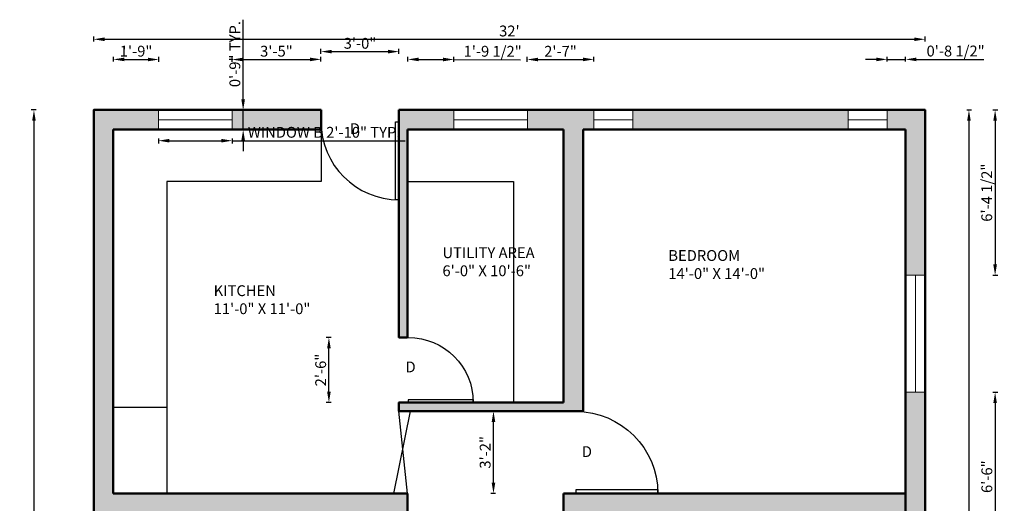
# Model space of a CAD drawing. Units: inches. Extents: x -41 to 449, y -587 to 56.
# Tile 2 of 2: x -32 to 422, y -167 to 56. Entities that reach past the tile are written whole.
import ezdxf

# ---------------------------------------------------------------- set-up
doc = ezdxf.new("R2010")
doc.units = ezdxf.units.IN
for name, color, linetype, lineweight in [('A-ANNO-DIMS', 2, 'Continuous', 18), ('A-ANNO-TEXT', 7, 'Continuous', 18), ('A-AREA-IDEN', 7, 'Continuous', 25), ('A-DOOR', 3, 'Continuous', 25), ('A-FLOR-CASE', 8, 'Continuous', 25), ('A-GLAZ', 4, 'Continuous', 18), ('A-WALL', 7, 'Continuous', 50), ('A-WALL-PATT', 252, 'Continuous', 13)]:
    doc.layers.add(name, color=color, linetype=linetype, lineweight=lineweight)
doc.styles.get("Standard").update_dxf_attribs({"font": 'arial.ttf'})
doc.dimstyles.new('ISO-25', dxfattribs={"dimtxt": 5, "dimasz": 5, "dimexe": 1.25, "dimexo": 0.625, "dimtad": 1, "dimlunit": 3, "dimtxsty": 'Standard', "dimcen": 2.5, "dimadec": 0, "dimazin": 0, "dimtfac": 1, "dimtmove": 0, "dimatfit": 3, "dimfxl": 1, "dimfxlon": 1, "dimarcsym": 0})

# ---------------------------------------------------------------- blocks, each defined once
blk = doc.blocks.new('*U2')
for p, q in [((0, 0), (0, -6)), ((40, 0), (40, -6))]:
    blk.add_line(p, q)
blk.add_lwpolyline([(0, 0), (0, 40), (1.75, 40), (1.75, 0)], close=True)
blk.add_arc((0, 0), 40, 0, 90)
blk = doc.blocks.new('*D3')
at = {"layer": 'A-ANNO-DIMS', "color": 0, "lineweight": -2, "transparency": 16777216}
for p, q in [((1.69, 45.8), (1.69, 48.05)), ((6.69, 46.8), (380.69, 46.8)), ((385.69, 45.8), (385.69, 48.05))]:
    blk.add_line(p, q, dxfattribs=at)
at = {"layer": 'A-ANNO-DIMS', "color": 0, "transparency": 16777216}
for points in [[(6.69, 47.63), (6.69, 45.97), (1.69, 46.8)], [(380.69, 47.63), (380.69, 45.97), (385.69, 46.8)]]:
    blk.add_solid(points, dxfattribs=at)
at = {"layer": 'Defpoints', "color": 0, "transparency": 16777216}
for p in [(385.69, 46.8), (1.69, 14.17), (385.69, 14.17)]:
    blk.add_point(p, dxfattribs=at)
at = {"layer": 'A-ANNO-DIMS', "color": 0, "transparency": 16777216, "insert": (193.69, 49.98), "char_height": 5, "attachment_point": 5}
blk.add_mtext("32'", dxfattribs=at)
blk = doc.blocks.new('*D4')
at = {"layer": 'A-ANNO-DIMS', "color": 0, "lineweight": -2, "transparency": 16777216}
for p, q in [((404.95, 14.17), (407.2, 14.17)), ((405.95, 9.17), (405.95, -524.83)), ((404.95, -529.83), (407.2, -529.83))]:
    blk.add_line(p, q, dxfattribs=at)
at = {"layer": 'A-ANNO-DIMS', "color": 0, "transparency": 16777216}
for points in [[(405.11, 9.17), (406.78, 9.17), (405.95, 14.17)], [(405.11, -524.83), (406.78, -524.83), (405.95, -529.83)]]:
    blk.add_solid(points, dxfattribs=at)
at = {"layer": 'Defpoints', "color": 0, "transparency": 16777216}
for p in [(385.69, 14.17), (385.69, -529.83), (405.95, -529.83)]:
    blk.add_point(p, dxfattribs=at)
at = {"layer": 'A-ANNO-DIMS', "color": 0, "transparency": 16777216, "insert": (402.78, -257.83), "char_height": 5, "attachment_point": 5, "rotation": 90}
blk.add_mtext('45\'-4"', dxfattribs=at)
blk = doc.blocks.new('*D5')
at = {"layer": 'A-ANNO-DIMS', "color": 0, "lineweight": -2, "transparency": 16777216}
for p, q in [((-24.91, 14.17), (-27.16, 14.17)), ((-25.91, 9.17), (-25.91, -454.83)), ((-24.91, -459.83), (-27.16, -459.83))]:
    blk.add_line(p, q, dxfattribs=at)
at = {"layer": 'A-ANNO-DIMS', "color": 0, "transparency": 16777216}
for points in [[(-26.74, 9.17), (-25.07, 9.17), (-25.91, 14.17)], [(-26.74, -454.83), (-25.07, -454.83), (-25.91, -459.83)]]:
    blk.add_solid(points, dxfattribs=at)
at = {"layer": 'Defpoints', "color": 0, "transparency": 16777216}
for p in [(1.69, 14.17), (-25.91, -459.83), (1.69, -459.83)]:
    blk.add_point(p, dxfattribs=at)
at = {"layer": 'A-ANNO-DIMS', "color": 0, "transparency": 16777216, "insert": (-29.09, -222.83), "char_height": 5, "attachment_point": 5, "rotation": 90}
blk.add_mtext('39\'-6"', dxfattribs=at)
blk = doc.blocks.new('WIN-54IN')
blk.add_line((4.5, 54), (4.5, 0))
blk.add_lwpolyline([(0, 54), (9, 54), (9, 0), (0, 0)], close=True)
blk = doc.blocks.new('WIN-34IN')
blk.add_line((0, 4.5), (34, 4.5))
blk.add_lwpolyline([(0, 9), (34, 9), (34, 0), (0, 0)], close=True)
blk = doc.blocks.new('WIN-18IN')
blk.add_line((0, 4.5), (18, 4.5))
blk.add_lwpolyline([(0, 9), (18, 9), (18, 0), (0, 0)], close=True)
blk = doc.blocks.new('*D14')
at = {"layer": 'A-ANNO-DIMS', "color": 0, "lineweight": -2, "transparency": 16777216}
for p, q in [((31.62, 1), (31.62, -1.25)), ((36.62, 0), (60.62, 0)), ((65.62, 1), (65.62, -1.25)), ((65.62, 0), (145.62, 0))]:
    blk.add_line(p, q, dxfattribs=at)
at = {"layer": 'A-ANNO-DIMS', "color": 0, "transparency": 16777216}
for points in [[(36.62, 0.84), (36.62, -0.83), (31.62, 0)], [(60.62, 0.84), (60.62, -0.83), (65.62, 0)]]:
    blk.add_solid(points, dxfattribs=at)
at = {"layer": 'Defpoints', "color": 0, "transparency": 16777216}
for p in [(31.62, 5.1), (65.62, 5.1), (65.62, 0)]:
    blk.add_point(p, dxfattribs=at)
at = {"layer": 'A-ANNO-DIMS', "color": 0, "transparency": 16777216, "insert": (108.12, 3.22), "char_height": 5, "attachment_point": 5}
blk.add_mtext('WINDOW B 2\'-10" TYP.', dxfattribs=at)
blk = doc.blocks.new('*D15')
at = {"layer": 'A-ANNO-DIMS', "color": 0, "lineweight": -2, "transparency": 16777216}
for p, q in [((70.72, 19.1), (70.72, 55.83)), ((69.72, 14.1), (71.97, 14.1)), ((70.72, 5.1), (70.72, 14.1)), ((69.72, 5.1), (71.97, 5.1)), ((70.72, 0.1), (70.72, -4.9))]:
    blk.add_line(p, q, dxfattribs=at)
at = {"layer": 'A-ANNO-DIMS', "color": 0, "transparency": 16777216}
for points in [[(69.89, 19.1), (71.55, 19.1), (70.72, 14.1)], [(69.89, 0.1), (71.55, 0.1), (70.72, 5.1)]]:
    blk.add_solid(points, dxfattribs=at)
at = {"layer": 'Defpoints', "color": 0, "transparency": 16777216}
for p in [(65.62, 14.1), (70.72, 14.1), (65.62, 5.1)]:
    blk.add_point(p, dxfattribs=at)
at = {"layer": 'A-ANNO-DIMS', "color": 0, "transparency": 16777216, "insert": (67.54, 39.97), "char_height": 5, "attachment_point": 5, "rotation": 90}
blk.add_mtext('0\'-9" TYP.', dxfattribs=at)
blk = doc.blocks.new('*D18')
at = {"layer": 'A-ANNO-DIMS', "color": 0, "lineweight": -2, "transparency": 16777216}
for p, q in [((10.79, 36.52), (10.8, 38.77)), ((15.79, 37.5), (26.72, 37.47)), ((31.71, 36.45), (31.72, 38.7))]:
    blk.add_line(p, q, dxfattribs=at)
at = {"layer": 'A-ANNO-DIMS', "color": 0, "transparency": 16777216}
for points in [[(15.79, 38.33), (15.79, 36.67), (10.79, 37.52)], [(26.72, 38.3), (26.71, 36.63), (31.72, 37.45)]]:
    blk.add_solid(points, dxfattribs=at)
at = {"layer": 'Defpoints', "color": 0, "transparency": 16777216}
for p in [(31.72, 37.45), (10.69, 5.17), (31.62, 5.1)]:
    blk.add_point(p, dxfattribs=at)
at = {"layer": 'A-ANNO-DIMS', "color": 0, "transparency": 16777216, "insert": (21.26, 40.66), "char_height": 5, "attachment_point": 5, "rotation": 359.828}
blk.add_mtext('1\'-9"', dxfattribs=at)
blk = doc.blocks.new('*D19')
at = {"layer": 'A-ANNO-DIMS', "color": 0, "lineweight": -2, "transparency": 16777216}
for p, q in [((65.57, 36.45), (65.57, 38.7)), ((70.57, 37.46), (101.65, 37.51)), ((106.65, 36.52), (106.64, 38.77))]:
    blk.add_line(p, q, dxfattribs=at)
at = {"layer": 'A-ANNO-DIMS', "color": 0, "transparency": 16777216}
for points in [[(70.57, 38.29), (70.57, 36.63), (65.57, 37.45)], [(101.64, 38.34), (101.65, 36.67), (106.65, 37.52)]]:
    blk.add_solid(points, dxfattribs=at)
at = {"layer": 'Defpoints', "color": 0, "transparency": 16777216}
for p in [(106.65, 37.52), (65.62, 5.1), (106.69, 5.17)]:
    blk.add_point(p, dxfattribs=at)
at = {"layer": 'A-ANNO-DIMS', "color": 0, "transparency": 16777216, "insert": (86.1, 40.66), "char_height": 5, "attachment_point": 5, "rotation": 0.0876}
blk.add_mtext('3\'-5"', dxfattribs=at)
blk = doc.blocks.new('*D20')
at = {"layer": 'A-ANNO-DIMS', "color": 0, "lineweight": -2, "transparency": 16777216}
for p, q in [((106.67, 40.11), (106.67, 42.36)), ((111.67, 41.11), (137.69, 41.11)), ((142.69, 40.11), (142.69, 42.36))]:
    blk.add_line(p, q, dxfattribs=at)
at = {"layer": 'A-ANNO-DIMS', "color": 0, "transparency": 16777216}
for points in [[(111.67, 41.95), (111.67, 40.28), (106.67, 41.11)], [(137.69, 41.95), (137.69, 40.28), (142.69, 41.11)]]:
    blk.add_solid(points, dxfattribs=at)
at = {"layer": 'Defpoints', "color": 0, "transparency": 16777216}
for p in [(142.69, 41.11), (106.67, 8.76), (142.69, 8.76)]:
    blk.add_point(p, dxfattribs=at)
at = {"layer": 'A-ANNO-DIMS', "color": 0, "transparency": 16777216, "insert": (124.68, 44.29), "char_height": 5, "attachment_point": 5}
blk.add_mtext('3\'-0"', dxfattribs=at)
blk = doc.blocks.new('*D21')
at = {"layer": 'A-ANNO-DIMS', "color": 0, "lineweight": -2, "transparency": 16777216}
for p, q in [((146.79, 36.52), (146.79, 38.77)), ((151.79, 37.5), (163.09, 37.47)), ((168.09, 36.45), (168.09, 38.7)), ((168.09, 37.45), (198.81, 37.36))]:
    blk.add_line(p, q, dxfattribs=at)
at = {"layer": 'A-ANNO-DIMS', "color": 0, "transparency": 16777216}
for points in [[(151.79, 38.33), (151.79, 36.67), (146.79, 37.52)], [(163.09, 38.3), (163.09, 36.63), (168.09, 37.45)]]:
    blk.add_solid(points, dxfattribs=at)
at = {"layer": 'Defpoints', "color": 0, "transparency": 16777216}
for p in [(168.09, 37.45), (146.69, 5.17), (167.99, 5.1)]:
    blk.add_point(p, dxfattribs=at)
at = {"layer": 'A-ANNO-DIMS', "color": 0, "transparency": 16777216, "insert": (185.96, 40.61), "char_height": 5, "attachment_point": 5, "rotation": 359.831}
blk.add_mtext('1\'-9 1/2"', dxfattribs=at)
blk = doc.blocks.new('*D22')
at = {"layer": 'A-ANNO-DIMS', "color": 0, "lineweight": -2, "transparency": 16777216}
for p, q in [((201.93, 36.45), (201.92, 38.7)), ((206.93, 37.46), (227.69, 37.51)), ((232.69, 36.52), (232.69, 38.77))]:
    blk.add_line(p, q, dxfattribs=at)
at = {"layer": 'A-ANNO-DIMS', "color": 0, "transparency": 16777216}
for points in [[(206.93, 38.3), (206.93, 36.63), (201.93, 37.45)], [(227.69, 38.34), (227.69, 36.67), (232.69, 37.52)]]:
    blk.add_solid(points, dxfattribs=at)
at = {"layer": 'Defpoints', "color": 0, "transparency": 16777216}
for p in [(232.69, 37.52), (201.99, 5.1), (232.76, 5.17)]:
    blk.add_point(p, dxfattribs=at)
at = {"layer": 'A-ANNO-DIMS', "color": 0, "transparency": 16777216, "insert": (217.3, 40.62), "char_height": 5, "attachment_point": 5, "rotation": 0.117}
blk.add_mtext('2\'-7"', dxfattribs=at)
blk = doc.blocks.new('*D23')
at = {"layer": 'A-ANNO-DIMS', "color": 0, "lineweight": -2, "transparency": 16777216}
for p, q in [((363.17, 37.52), (358.17, 37.52)), ((368.17, 36.52), (368.17, 38.77)), ((368.17, 37.52), (376.69, 37.52)), ((376.69, 36.52), (376.69, 38.77)), ((381.69, 37.52), (412.89, 37.52))]:
    blk.add_line(p, q, dxfattribs=at)
at = {"layer": 'A-ANNO-DIMS', "color": 0, "transparency": 16777216}
for points in [[(363.17, 38.35), (363.17, 36.68), (368.17, 37.52)], [(381.69, 38.35), (381.69, 36.68), (376.69, 37.52)]]:
    blk.add_solid(points, dxfattribs=at)
at = {"layer": 'Defpoints', "color": 0, "transparency": 16777216}
for p in [(376.69, 37.52), (368.17, 5.17), (376.69, 5.17)]:
    blk.add_point(p, dxfattribs=at)
at = {"layer": 'A-ANNO-DIMS', "color": 0, "transparency": 16777216, "insert": (399.79, 40.73), "char_height": 5, "attachment_point": 5}
blk.add_mtext('0\'-8 1/2"', dxfattribs=at)
blk = doc.blocks.new('*D24')
at = {"layer": 'A-ANNO-DIMS', "color": 0, "lineweight": -2, "transparency": 16777216}
for p, q in [((417.04, 14.17), (419.29, 14.17)), ((418.04, 9.17), (418.04, -57.12)), ((417.04, -62.12), (419.29, -62.12))]:
    blk.add_line(p, q, dxfattribs=at)
at = {"layer": 'A-ANNO-DIMS', "color": 0, "transparency": 16777216}
for points in [[(417.21, 9.17), (418.88, 9.17), (418.04, 14.17)], [(417.21, -57.12), (418.88, -57.12), (418.04, -62.12)]]:
    blk.add_solid(points, dxfattribs=at)
at = {"layer": 'Defpoints', "color": 0, "transparency": 16777216}
for p in [(385.69, 14.17), (385.69, -62.12), (418.04, -62.12)]:
    blk.add_point(p, dxfattribs=at)
at = {"layer": 'A-ANNO-DIMS', "color": 0, "transparency": 16777216, "insert": (414.83, -23.98), "char_height": 5, "attachment_point": 5, "rotation": 90}
blk.add_mtext('6\'-4 1/2"', dxfattribs=at)
blk = doc.blocks.new('*D25')
at = {"layer": 'A-ANNO-DIMS', "color": 0, "lineweight": -2, "transparency": 16777216}
for p, q in [((417.04, -116.12), (419.29, -116.12)), ((418.04, -121.12), (418.04, -189)), ((417.04, -194), (419.29, -194))]:
    blk.add_line(p, q, dxfattribs=at)
at = {"layer": 'A-ANNO-DIMS', "color": 0, "transparency": 16777216}
for points in [[(417.21, -121.12), (418.88, -121.12), (418.04, -116.12)], [(417.21, -189), (418.88, -189), (418.04, -194)]]:
    blk.add_solid(points, dxfattribs=at)
at = {"layer": 'Defpoints', "color": 0, "transparency": 16777216}
for p in [(385.69, -116.12), (385.69, -194), (418.04, -194)]:
    blk.add_point(p, dxfattribs=at)
at = {"layer": 'A-ANNO-DIMS', "color": 0, "transparency": 16777216, "insert": (414.87, -155.06), "char_height": 5, "attachment_point": 5, "rotation": 90}
blk.add_mtext('6\'-6"', dxfattribs=at)
blk = doc.blocks.new('*D35')
at = {"layer": 'A-ANNO-DIMS', "color": 0, "lineweight": -2, "transparency": 16777216}
for p, q in [((111.34, -90.83), (109.09, -90.83)), ((110.34, -115.83), (110.34, -95.83)), ((111.34, -120.83), (109.09, -120.83))]:
    blk.add_line(p, q, dxfattribs=at)
at = {"layer": 'A-ANNO-DIMS', "color": 0, "transparency": 16777216}
for points in [[(109.51, -95.83), (111.18, -95.83), (110.34, -90.83)], [(109.51, -115.83), (111.18, -115.83), (110.34, -120.83)]]:
    blk.add_solid(points, dxfattribs=at)
at = {"layer": 'Defpoints', "color": 0, "transparency": 16777216}
for p in [(110.34, -90.83), (142.69, -90.83), (142.69, -120.83)]:
    blk.add_point(p, dxfattribs=at)
at = {"layer": 'A-ANNO-DIMS', "color": 0, "transparency": 16777216, "insert": (107.17, -105.83), "char_height": 5, "attachment_point": 5, "rotation": 90}
blk.add_mtext('2\'-6"', dxfattribs=at)
blk = doc.blocks.new('*D36')
at = {"layer": 'A-ANNO-DIMS', "color": 0, "lineweight": -2, "transparency": 16777216}
for p, q in [((187.34, -124.83), (185.09, -124.83)), ((186.34, -157.83), (186.34, -129.83)), ((187.34, -162.83), (185.09, -162.83))]:
    blk.add_line(p, q, dxfattribs=at)
at = {"layer": 'A-ANNO-DIMS', "color": 0, "transparency": 16777216}
for points in [[(185.51, -129.83), (187.18, -129.83), (186.34, -124.83)], [(185.51, -157.83), (187.18, -157.83), (186.34, -162.83)]]:
    blk.add_solid(points, dxfattribs=at)
at = {"layer": 'Defpoints', "color": 0, "transparency": 16777216}
for p in [(186.34, -124.83), (218.69, -124.83), (218.69, -162.83)]:
    blk.add_point(p, dxfattribs=at)
at = {"layer": 'A-ANNO-DIMS', "color": 0, "transparency": 16777216, "insert": (183.16, -143.83), "char_height": 5, "attachment_point": 5, "rotation": 90}
blk.add_mtext('3\'-2"', dxfattribs=at)

msp = doc.modelspace()

# ---------------------------------------------------------------- hatches: boundary and pattern name
at = {"layer": 'A-WALL-PATT'}
h = msp.add_hatch(color=256, dxfattribs=at)
h.dxf.hatch_style = 1
h.paths.add_polyline_path([(106.669, 14.166), (65.62, 14.166), (65.62, 5.166), (106.695, 5.166), (106.695, 7.401, -0.0094448), (106.669, 8.762)], flags=17)
h.paths.add_polyline_path([(31.62, 14.166), (1.695, 14.166), (1.695, -216.327), (10.695, -216.327), (10.695, -171.834), (146.695, -171.834), (146.695, -162.834), (10.695, -162.834), (10.695, 5.166), (31.62, 5.166)])
h.paths.add_polyline_path([(167.994, 14.166), (142.695, 14.166), (142.695, 8.762), (142.695, -27.264), (142.695, -90.806), (146.695, -90.806), (146.695, 5.166), (167.994, 5.166)])
h.paths.add_polyline_path([(232.757, 14.166), (201.994, 14.166), (201.994, 5.166), (218.695, 5.166), (218.695, -120.834), (142.695, -120.834), (142.695, -124.834), (146.695, -124.834), (218.695, -124.834), (227.695, -124.834), (227.695, 5.166), (232.757, 5.166)])
h.paths.add_polyline_path([(350.174, 14.166), (250.757, 14.166), (250.757, 5.166), (350.174, 5.166)])
h.paths.add_polyline_path([(385.695, 14.166), (368.174, 14.166), (368.174, 5.166), (376.695, 5.166), (376.695, -62.119), (385.695, -62.119)])
h.paths.add_polyline_path([(385.695, -116.119), (376.695, -116.119), (376.695, -194.002), (385.695, -194.002)])
h.paths.add_polyline_path([(376.695, -162.834), (227.695, -162.834), (224.376, -162.834), (218.695, -162.834), (218.695, -271.834), (227.695, -271.834), (376.695, -271.834), (376.695, -267.834), (227.695, -267.834), (227.695, -171.834), (376.695, -171.834)])
h.paths.add_polyline_path([(385.695, -228.002), (376.695, -228.002), (376.695, -295.429), (385.695, -295.429)])
h.paths.add_polyline_path([(385.695, -329.429), (376.695, -329.429), (376.695, -394.588), (385.695, -394.588)])
h.paths.add_polyline_path([(376.695, -343.834), (317.695, -343.834), (317.695, -343.936), (282.107, -343.936), (276.769, -343.936), (263.368, -343.835), (263.368, -349.185, -0.0248206), (263.192, -352.72), (263.192, -352.834), (376.695, -352.834)])
h.paths.add_polyline_path([(280.695, -271.834), (276.695, -271.834), (276.695, -308.243), (280.695, -308.243)])
h.paths.add_polyline_path([(227.695, -343.834), (218.695, -343.834), (218.695, -432.415), (218.799, -432.415), (218.799, -456.484), (218.799, -460.095), (218.695, -520.834), (218.695, -529.834), (231.695, -529.834), (231.695, -520.834), (227.695, -520.834)])
h.paths.add_polyline_path([(354.695, -520.834), (249.695, -520.834), (249.695, -529.834), (354.695, -529.834)])
h.paths.add_polyline_path([(385.695, -448.588), (376.695, -448.588), (376.695, -520.834), (372.695, -520.834), (372.695, -529.834), (385.695, -529.834)])
h.paths.add_polyline_path([(170.695, -456.353), (170.695, -450.834), (106.802, -450.834), (106.802, -459.834), (170.695, -459.834)])
h.paths.add_polyline_path([(52.802, -450.834), (10.695, -450.834), (10.695, -423.396), (1.695, -423.396), (1.695, -459.834), (52.802, -459.834)])
h.paths.add_polyline_path([(10.695, -270.327), (1.695, -270.327), (1.695, -369.396), (10.695, -369.396)])

# ---------------------------------------------------------------- linework, layer by layer
at = {"layer": 'A-DOOR'}
for p, q in [((140.3, -162.834), (148.006, -124.834)), ((146.695, -162.834), (142.695, -124.834))]:
    msp.add_line(p, q, dxfattribs=at)
at = {"layer": 'A-FLOR-CASE'}
for p, q in [((106.695, 5.166), (106.695, -18.834)), ((106.695, -18.834), (35.445, -18.834)), ((35.445, -18.834), (35.445, -162.834)), ((146.695, -18.834), (195.568, -18.834)), ((195.568, -18.834), (195.568, -120.834)), ((10.695, -122.956), (35.445, -122.956))]:
    msp.add_line(p, q, dxfattribs=at)
at = {"layer": 'A-WALL'}
for p, q in [((106.695, 5.166), (106.695, 14.166)), ((142.695, -90.834), (142.695, 14.166)), ((10.695, 5.166), (106.695, 5.166)), ((10.695, -162.834), (10.695, 5.166)), ((146.695, 5.166), (218.695, 5.166)), ((146.695, -90.834), (146.695, 5.166)), ((146.695, 5.166), (218.695, 5.166)), ((218.695, -120.834), (218.695, 5.166)), ((227.695, 5.166), (376.695, 5.166)), ((227.695, 5.166), (376.695, 5.166)), ((227.695, -124.834), (227.695, 5.166)), ((376.695, 5.166), (376.695, -520.834)), ((146.695, -90.834), (142.695, -90.834)), ((142.695, -120.834), (218.695, -120.834)), ((142.695, -124.834), (142.695, -120.834)), ((146.695, -124.834), (142.695, -124.834)), ((146.695, -124.834), (218.695, -124.834)), ((218.695, -124.834), (227.695, -124.834)), ((10.695, -162.834), (146.695, -162.834)), ((146.695, -171.834), (146.695, -162.834)), ((227.695, -162.834), (218.695, -162.834)), ((218.695, -271.834), (218.695, -162.834)), ((227.695, -162.834), (376.695, -162.834))]:
    msp.add_line(p, q, dxfattribs=at)
msp.add_lwpolyline([(142.695, 14.166), (385.695, 14.166), (385.695, -529.834), (1.695, -529.834), (1.695, 14.166), (106.695, 14.166)], dxfattribs=at)

# ---------------------------------------------------------------- block references
at = {"layer": 'A-DOOR'}
for p, xscale, yscale, zscale, rotation in [((142.695, 8.762), 0.9006426185907889, 0.9006426185907889, 0.9006426185907889, 180), ((146.976, -120.834), -0.7506909712206064, 0.7506909712206064, 0.7506909712206064, 270), ((224.376, -162.834), -0.946864636577651, 0.946864636577651, 0.946864636577651, 270)]:
    msp.add_blockref('*U2', p, dxfattribs=dict(at, xscale=xscale, yscale=yscale, zscale=zscale, rotation=rotation))
at = {"layer": 'A-GLAZ'}
for name, p in [('WIN-34IN', (31.62, 5.103)), ('WIN-34IN', (167.994, 5.103)), ('WIN-18IN', (232.757, 5.166)), ('WIN-18IN', (350.174, 5.166)), ('WIN-54IN', (376.695, -116.119))]:
    msp.add_blockref(name, p, dxfattribs=at)

# ---------------------------------------------------------------- texts
at = {"layer": 'A-ANNO-TEXT', "char_height": 5, "attachment_point": 1}
for width, insert in [(9.69444, (120.022, 8.076)), (11.71258, (145.704, -101.917)), (8.27436, (227.157, -140.992))]:
    msp.add_mtext_dynamic_manual_height_columns('D', width=width, gutter_width=12.5, heights=[0], dxfattribs=dict(at, insert=insert))
at = {"layer": 'A-AREA-IDEN', "char_height": 5, "attachment_point": 1}
for s, width, insert in [('UTILITY AREA\\P6\'-0" X 10\'-6"', 55.92782, (162.767, -49.199)), ('BEDROOM\\P14\'-0" X 14\'-0"', 71.55561, (267.093, -50.487)), ('KITCHEN\\P11\'-0" X 11\'-0"', 63.39929, (57.101, -66.721))]:
    msp.add_mtext_dynamic_manual_height_columns(s, width=width, gutter_width=12.5, heights=[0], dxfattribs=dict(at, insert=insert))

# ---------------------------------------------------------------- dimensions: what is measured, and where the dimension line sits
at = {"layer": 'A-ANNO-DIMS'}
dim = msp.add_linear_dim(base=(70.72, 14.103), p1=(65.62, 5.103), p2=(65.62, 14.103), angle=90, text='<> TYP.', dimstyle='ISO-25', override={"dimdec": 1, "dimlfac": 1, "dimrnd": 0, "dimzin": 1, "dimdsep": 46, "dimlunit": 4, "dimfrac": 2}, dxfattribs=at)
dim.commit()
dim.dimension.update_dxf_attribs({"geometry": '*D15', "text_midpoint": (67.542, 39.967)})
for base, p1, p2, override, picture, middle in [((385.695, 46.801), (1.695, 14.166), (385.695, 14.166), {"dimclrd": 0, "dimclre": 0, "dimclrt": 0}, '*D3', (193.695, 49.981)), ((142.695, 41.112), (106.669, 8.762), (142.695, 8.762), {"dimdec": 1, "dimlfac": 1, "dimrnd": 0, "dimzin": 1, "dimdsep": 46, "dimlunit": 4, "dimfrac": 2}, '*D20', (124.682, 44.292))]:
    dim = msp.add_linear_dim(base=base, p1=p1, p2=p2, dimstyle='ISO-25', override=override, dxfattribs=at)
    dim.commit()
    dim.dimension.update_dxf_attribs({"geometry": picture, "text_midpoint": middle})
for base, p1, p2, angle, override, picture, middle in [((168.089, 37.453), (146.695, 5.166), (167.994, 5.103), 359.83098, {"dimdec": 1, "dimlfac": 1, "dimrnd": 0, "dimzin": 1, "dimdsep": 46, "dimlunit": 4, "dimfrac": 2}, '*D21', (185.959, 40.611)), ((376.695, 37.516), (368.174, 5.166), (376.695, 5.166), 0, {"dimdec": 1, "dimlfac": 1, "dimrnd": 0, "dimzin": 1, "dimdsep": 46, "dimlunit": 4, "dimfrac": 2}, '*D23', (399.791, 40.726)), ((31.717, 37.453), (10.695, 5.166), (31.62, 5.103), 359.82796, {"dimdec": 1, "dimlfac": 1, "dimrnd": 0, "dimzin": 1, "dimdsep": 46, "dimlunit": 4, "dimfrac": 2}, '*D18', (21.264, 40.662)), ((106.645, 37.516), (65.62, 5.103), (106.695, 5.166), 0.08764, {"dimdec": 1, "dimlfac": 1, "dimrnd": 0, "dimzin": 1, "dimdsep": 46, "dimlunit": 4, "dimfrac": 2}, '*D19', (86.103, 40.664)), ((232.691, 37.516), (201.994, 5.103), (232.757, 5.166), 0.11702, {"dimdec": 1, "dimlfac": 1, "dimrnd": 0, "dimzin": 1, "dimdsep": 46, "dimlunit": 4, "dimfrac": 2}, '*D22', (217.303, 40.62)), ((-25.907, -459.834), (1.695, 14.166), (1.695, -459.834), 90, {"dimclrd": 0, "dimclre": 0, "dimclrt": 0}, '*D5', (-29.087, -222.834)), ((405.948, -529.834), (385.695, 14.166), (385.695, -529.834), 90, {"dimclrd": 0, "dimclre": 0, "dimclrt": 0}, '*D4', (402.781, -257.834)), ((418.045, -62.119), (385.695, 14.166), (385.695, -62.119), 270, {"dimdec": 1, "dimlfac": 1, "dimrnd": 0, "dimzin": 1, "dimdsep": 46, "dimlunit": 4, "dimfrac": 2}, '*D24', (414.834, -23.976)), ((110.345, -90.834), (142.695, -120.834), (142.695, -90.834), 90, {"dimdec": 1, "dimlfac": 1, "dimrnd": 0, "dimzin": 1, "dimdsep": 46, "dimlunit": 4, "dimfrac": 2}, '*D35', (107.167, -105.834)), ((418.045, -194.002), (385.695, -116.119), (385.695, -194.002), 270, {"dimdec": 1, "dimlfac": 1, "dimrnd": 0, "dimzin": 1, "dimdsep": 46, "dimlunit": 4, "dimfrac": 2}, '*D25', (414.867, -155.06)), ((186.345, -124.834), (218.695, -162.834), (218.695, -124.834), 90, {"dimdec": 1, "dimlfac": 1, "dimrnd": 0, "dimzin": 1, "dimdsep": 46, "dimlunit": 4, "dimfrac": 2}, '*D36', (183.165, -143.834))]:
    dim = msp.add_linear_dim(base=base, p1=p1, p2=p2, angle=angle, dimstyle='ISO-25', override=override, dxfattribs=at)
    dim.commit()
    dim.dimension.update_dxf_attribs({"geometry": picture, "text_midpoint": middle})
dim = msp.add_linear_dim(base=(65.62, 0.003), p1=(31.62, 5.103), p2=(65.62, 5.103), text='WINDOW B <> TYP.', dimstyle='ISO-25', override={"dimdec": 1, "dimlfac": 1, "dimrnd": 0, "dimzin": 1, "dimdsep": 46, "dimlunit": 4, "dimfrac": 2}, dxfattribs=at)
dim.commit()
dim.dimension.update_dxf_attribs({"geometry": '*D14', "text_midpoint": (108.122, 3.215)})

doc.saveas('drawing.dxf')
